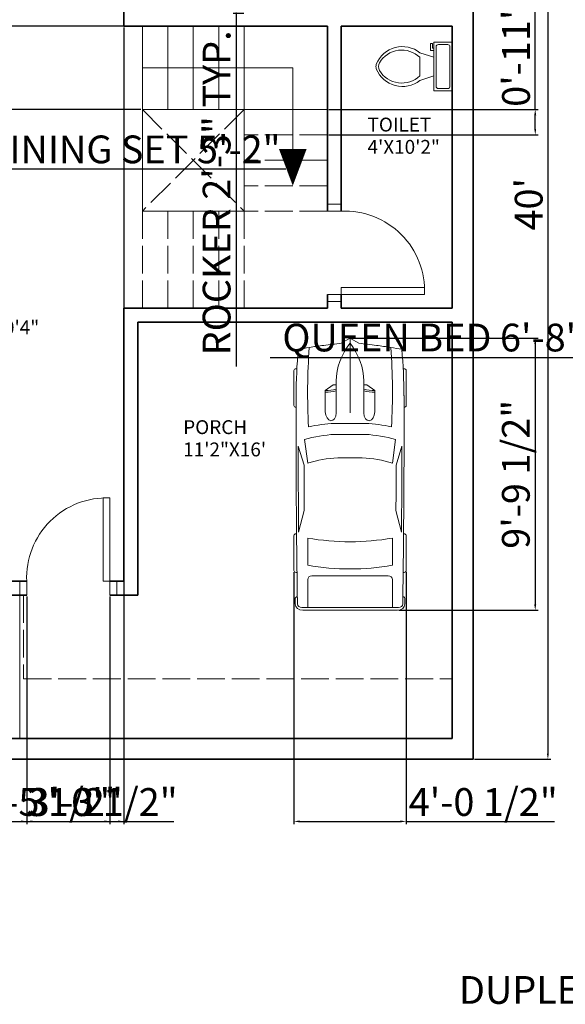
# Model space of a CAD drawing. Units: inches. Extents: x 2446 to 3341, y 462 to 1195.
# Tile 2 of 6: x 2649 to 2884, y 462 to 888. Entities that reach past the tile are written whole.
import ezdxf

# ---------------------------------------------------------------- set-up
doc = ezdxf.new("R2010")
doc.units = ezdxf.units.IN
doc.linetypes.add('ACAD_ISO02W100', pattern=[15, 12, -3])
for name, color, linetype, lineweight in [('A-ANNO-DIMS', 2, 'Continuous', 18), ('A-ANNO-TEXT', 7, 'Continuous', 25), ('A-AREA-IDEN', 7, 'Continuous', 18), ('A-DOOR', 4, 'Continuous', 18), ('A-FLOR-FIXT', 9, 'Continuous', 18), ('A-FLOR-HIDN', 8, 'ACAD_ISO02W100', 18), ('A-FLOR-STRS', 7, 'Continuous', 18), ('A-FLOR-STRS-HIDN', 8, 'ACAD_ISO02W100', 18), ('A-WALL', 7, 'Continuous', 35), ('C-PROP', 7, 'Continuous', 35), ('C-SITE-VEHC', 8, 'Continuous', 13), ('L-PLNT', 3, 'Continuous', 18)]:
    doc.layers.add(name, color=color, linetype=linetype, lineweight=lineweight)
doc.styles.get("Standard").update_dxf_attribs({"font": 'arial.ttf'})
doc.dimstyles.new('ISO-25', dxfattribs={"dimtxt": 12, "dimasz": 2.5, "dimexe": 1.25, "dimexo": 0.625, "dimtad": 1, "dimdec": 1, "dimlunit": 3, "dimtxsty": 'Standard', "dimcen": 2.5, "dimadec": 0, "dimazin": 0, "dimtfac": 1, "dimtdec": 1, "dimtmove": 0, "dimatfit": 3, "dimfxl": 1, "dimarcsym": 0})

# ---------------------------------------------------------------- blocks, each defined once
blk = doc.blocks.new('Toilet - top')
for p, q in [((9.5, -6), (9.5, -2)), ((-10, -8.5), (-8, -8.5)), ((-10, -9.5), (-10, -8.5)), ((-8, -8.5), (-8, -8)), ((-7, -8), (-7, -9.5)), ((-4, -8), (-6, -14)), ((4, -8), (6, -14)), ((-7, -9.5), (-10, -9.5)), ((4, -14), (-4, -14))]:
    blk.add_line(p, q)
blk.add_lwpolyline([(10.5, -8), (10.5, 0), (-10.5, 0), (-10.5, -8)], close=True)
for points in [[(-9.5, -2), (-9.5, -6)], [(8.5, -1), (-8.5, -1)], [(-8.5, -7), (8.5, -7)]]:
    blk.add_lwpolyline(points)
for centre, radius, start, end in [((-8.62, -1.88), 0.884, 81.8699, 188.1301), ((8.62, -1.88), 0.884, 351.8699, 98.1301), ((-8.62, -6.12), 0.884, 171.8699, 278.1301), ((8.62, -6.12), 0.884, 261.8699, 8.1301), ((3.52, -21.58), 12.17, 141.4691, 247.9714), ((4.2, -21.82), 11.33, 136.3677, 238.9468), ((-3.52, -21.58), 12.17, 292.0284, 38.5307), ((-4.2, -21.82), 11.33, 301.053, 43.6321), ((0, -27.88), 4, 245.7318, 294.2682), ((0, -29), 4, 254.8605, 285.1395)]:
    blk.add_arc(centre, radius, start, end)
blk = doc.blocks.new('*U14')
for p, q in [((21.1, 37.41), (21.1, 36.83)), ((46.55, 38.89), (22.35, 38.89)), ((47.8, 37.39), (47.8, 37.41)), ((87.99, 31.87), (74.76, 35.92)), ((134.31, 35.6), (119.29, 31.78)), ((135.45, 37.07), (135.45, 37.41)), ((136.7, 38.89), (160.9, 38.89)), ((162.15, 37.41), (162.15, 36.77)), ((70.03, 31.54), (86.41, 29.35)), ((138.42, 29.35), (157.25, 29.35)), ((186.47, 29.35), (167.01, 29.35)), ((186.47, -33.5), (186.47, 33.5)), ((188.4, -32.76), (188.4, 32.76)), ((164.52, 26.39), (164.52, -26.39)), ((32.27, 11.63), (36.13, 17.17)), ((36.13, 17.17), (50.94, 17.17)), ((29.77, 9.51), (51.68, 9.51)), ((32.12, 9.51), (32.12, 11.15)), ((58.92, -10.77), (58.92, 10.77)), ((66.55, -10.53), (66.55, 10.53)), ((82.74, 8.5), (82.74, -8.5)), ((186.47, -10.53), (186.47, 10.53)), ((3.27, 6.13), (0.1, 0.41)), ((0, 0), (51.68, 0)), ((0.1, -0.41), (3.27, -6.13)), ((29.77, -9.51), (51.68, -9.51)), ((32.12, -9.51), (32.12, -11.15)), ((32.27, -11.63), (36.13, -17.17)), ((36.13, -17.17), (50.94, -17.17)), ((86.41, -29.35), (70.03, -31.54)), ((87.99, -31.87), (74.76, -35.92)), ((134.31, -35.6), (119.29, -31.78)), ((157.25, -29.35), (138.42, -29.35)), ((167.01, -29.35), (186.47, -29.35)), ((21.1, -37.41), (21.1, -36.83)), ((46.55, -38.89), (22.35, -38.89)), ((47.8, -37.39), (47.8, -37.41)), ((135.45, -37.07), (135.45, -37.41)), ((136.7, -38.89), (160.9, -38.89)), ((162.15, -37.41), (162.15, -36.77))]:
    blk.add_line(p, q)
for centre, major_axis, ratio, start_param, end_param in [((266.03, -27.52), (0, 313.31), 0.842304, 1.367076, 1.39176), ((41.19, -490.86), (0, 528.23), 0.842304, 0.00281, 0.075598), ((22.35, 37.41), (0, -1.48), 0.842304, 3.141593, 4.712389), ((64.48, -10555.62), (0, 10593.03), 0.842304, -0.013397, 0.002797), ((46.55, 37.41), (0, 1.48), 0.842304, -1.570796, 0), ((64.48, -10555.62), (0, -10591.55), 0.842304, 3.133765, 3.140441), ((136.7, 37.41), (0, -1.48), 0.842304, 3.141593, 4.712389), ((160.9, 37.41), (0, 1.48), 0.842304, -1.570796, 0), ((180.63, 35.84), (0, 2.22), 0.842304, -0.013017, 1.249894), ((64.48, -10556.36), (0, 10595.31), 0.842304, -0.013397, -0.013017), ((183.98, 33.5), (0, -2.96), 0.842304, 1.570796, 3.128196), ((183.98, 32.76), (0, -5.25), 0.842304, 1.570796, 3.128196), ((259.18, -27.52), (0, -305.3), 0.842304, 4.528606, 4.561838), ((37.47, -593.96), (0, -623.33), 0.842304, 3.096046, 3.200911), ((134.4, 5.39), (0, -89.78), 0.842304, 4.449482, 4.652344), ((135.29, 5.39), (0, 81.77), 0.842304, 1.245306, 1.50788), ((149.6, 2.8), (0, -79.58), 0.842304, 4.372215, 4.640744), ((95.79, -3666.35), (0, -3698.24), 0.842304, 3.134049, 3.144098), ((17.08, 0), (0, 147.02), 0.842304, 4.511394, 4.913384), ((35.91, 0), (0, 147.02), 0.842304, 4.511394, 4.913384), ((167.01, 26.39), (0, 2.96), 0.842304, 0, 1.570796), ((-204.49, 52.4), (0, -250.96), 0.842304, 1.385369, 1.434372), ((13.04, 17.01), (0, 27.42), 0.842304, 4.435146, 4.718221), ((14.2, 17.01), (0, 27.42), 0.842304, 4.435146, 4.718221), ((50.79, 13.34), (6.34, -0.36), 0.603834, -1.395552, 1.581315), ((29.77, -46.66), (0, 56.17), 0.842304, 0, 0.590319), ((32.75, 11.15), (0, 0.74), 0.842304, 0.879714, 1.570796), ((0.62, 0), (0, -0.74), 0.842304, 4.131459, 5.293319), ((-204.49, -52.4), (0, 250.96), 0.842304, -1.434372, -1.385369), ((29.77, 46.66), (0, 56.17), 0.842304, 2.551274, 3.141593), ((32.75, -11.15), (0, -0.74), 0.842304, 4.712389, 5.403472), ((13.04, -17.01), (0, -27.42), 0.842304, 1.564964, 1.848039), ((14.2, -17.01), (0, -27.42), 0.842304, 1.564964, 1.848039), ((134.4, -5.39), (0, -89.78), 0.842304, -1.510751, -1.307889), ((135.29, -5.39), (0, -81.77), 0.842304, -1.50788, -1.245306), ((149.6, -2.8), (0, -79.58), 0.842304, -1.499151, -1.230623), ((259.18, 27.52), (0, 305.3), 0.842304, 1.721348, 1.754579), ((167.01, -26.39), (0, -2.96), 0.842304, 4.712389, 6.283185), ((266.03, 27.52), (0, 313.31), 0.842304, 1.749832, 1.774517), ((37.47, 593.96), (0, -623.33), 0.842304, -0.059319, 0.045547), ((95.79, 3666.35), (0, -3698.24), 0.842304, -0.002505, 0.007544), ((183.98, -33.5), (0, 2.96), 0.842304, 3.15499, 4.712389), ((183.98, -32.76), (0, -5.25), 0.842304, 0.013397, 1.570796), ((41.19, 490.86), (0, -528.23), 0.842304, -0.075598, -0.00281), ((22.35, -37.41), (0, 1.48), 0.842304, 1.570796, 3.141593), ((64.48, 10555.62), (0, 10593.03), 0.842304, 3.138796, 3.15499), ((46.55, -37.41), (0, -1.48), 0.842304, 0, 1.570796), ((64.48, 10555.62), (0, -10591.55), 0.842304, 0.001152, 0.007828), ((136.7, -37.41), (0, -1.48), 0.842304, -1.570796, 0), ((160.9, -37.41), (0, 1.48), 0.842304, 3.141593, 4.712389), ((180.63, -35.84), (0, -2.22), 0.842304, -1.249894, 0.013017), ((64.48, 10556.36), (0, 10595.31), 0.842304, 3.15461, 3.15499)]:
    blk.add_ellipse(centre, major_axis=major_axis, ratio=ratio, start_param=start_param, end_param=end_param)
at = {"extrusion": (0, 0, -1)}
blk.add_ellipse((50.79, -13.34), major_axis=(6.34, 0.36), ratio=0.603834, start_param=-1.395552, end_param=1.581315, dxfattribs=at)
blk = doc.blocks.new('*D18')
at = {"layer": 'A-ANNO-DIMS', "color": 0, "lineweight": -2, "transparency": 16777216}
for p, q in [((2845.24, 1047.97), (2878.2, 1047.97)), ((2876.95, 1045.47), (2876.95, 570.47)), ((2845.24, 567.97), (2878.2, 567.97))]:
    blk.add_line(p, q, dxfattribs=at)
at = {"layer": 'A-ANNO-DIMS', "color": 0, "transparency": 16777216}
for points in [[(2876.53, 1045.47), (2877.37, 1045.47), (2876.95, 1047.97)], [(2876.53, 570.47), (2877.37, 570.47), (2876.95, 567.97)]]:
    blk.add_solid(points, dxfattribs=at)
at = {"layer": 'Defpoints', "color": 0, "transparency": 16777216}
for p in [(2844.62, 1047.97), (2844.62, 567.97), (2876.95, 567.97)]:
    blk.add_point(p, dxfattribs=at)
at = {"layer": 'A-ANNO-DIMS', "color": 0, "transparency": 16777216, "insert": (2870.2, 807.97), "char_height": 12, "attachment_point": 5, "rotation": 90}
blk.add_mtext("40'", dxfattribs=at)
blk = doc.blocks.new('DOOR-SWING-36IN')
for p, q in [((6, 42), (0, 42)), ((6, 39), (0, 39)), ((6, 3), (0, 3)), ((6, 0), (0, 0))]:
    blk.add_line(p, q)
blk.add_lwpolyline([(6, 3), (42, 3), (42, 6), (6, 6)], close=True)
blk.add_arc((7.5, 4.5), 34.53, 357.5104, 92.4896)
blk = doc.blocks.new('*D29')
at = {"layer": 'A-ANNO-DIMS', "color": 0, "lineweight": -2, "transparency": 16777216}
for p, q in [((2937.19, 741.58), (2756.92, 741.58)), ((2937.19, 730.2), (2937.19, 742.83)), ((3014.69, 741.58), (2939.69, 741.58)), ((3017.19, 730.2), (3017.19, 742.83))]:
    blk.add_line(p, q, dxfattribs=at)
at = {"layer": 'A-ANNO-DIMS', "color": 0, "transparency": 16777216}
for points in [[(2939.69, 742), (2939.69, 741.16), (2937.19, 741.58)], [(3014.69, 742), (3014.69, 741.16), (3017.19, 741.58)]]:
    blk.add_solid(points, dxfattribs=at)
at = {"layer": 'Defpoints', "color": 0, "transparency": 16777216}
for p in [(2937.19, 741.58), (2937.19, 729.58), (3017.19, 729.58)]:
    blk.add_point(p, dxfattribs=at)
at = {"layer": 'A-ANNO-DIMS', "color": 0, "transparency": 16777216, "insert": (2845.81, 748.78), "char_height": 12, "attachment_point": 5}
blk.add_mtext('QUEEN BED 6\'-8" TYP.', dxfattribs=at)
blk = doc.blocks.new('*D33')
at = {"layer": 'A-ANNO-DIMS', "color": 0, "lineweight": -2, "transparency": 16777216}
for p, q in [((2745.53, 917.47), (2740.86, 917.47)), ((2742.11, 914.97), (2742.11, 892.97)), ((2745.53, 890.47), (2740.86, 890.47)), ((2742.11, 890.47), (2742.11, 737.82))]:
    blk.add_line(p, q, dxfattribs=at)
at = {"layer": 'A-ANNO-DIMS', "color": 0, "transparency": 16777216}
for points in [[(2741.69, 914.97), (2742.53, 914.97), (2742.11, 917.47)], [(2741.69, 892.97), (2742.53, 892.97), (2742.11, 890.47)]]:
    blk.add_solid(points, dxfattribs=at)
at = {"layer": 'Defpoints', "color": 0, "transparency": 16777216}
for p in [(2746.16, 917.47), (2742.11, 890.47), (2746.16, 890.47)]:
    blk.add_point(p, dxfattribs=at)
at = {"layer": 'A-ANNO-DIMS', "color": 0, "transparency": 16777216, "insert": (2735.27, 812.89), "char_height": 12, "attachment_point": 5, "rotation": 90}
blk.add_mtext('ROCKER 2\'-3" TYP.', dxfattribs=at)
blk = doc.blocks.new('*D53')
at = {"layer": 'A-ANNO-DIMS', "color": 0, "lineweight": -2, "transparency": 16777216}
for p, q in [((2566.04, 831.98), (2566.04, 822.05)), ((2628.06, 831.98), (2628.06, 822.05)), ((2568.54, 823.3), (2625.56, 823.3)), ((2628.06, 823.3), (2763.7, 823.3))]:
    blk.add_line(p, q, dxfattribs=at)
at = {"layer": 'A-ANNO-DIMS', "color": 0, "transparency": 16777216}
for points in [[(2568.54, 823.72), (2568.54, 822.89), (2566.04, 823.3)], [(2625.56, 823.72), (2625.56, 822.89), (2628.06, 823.3)]]:
    blk.add_solid(points, dxfattribs=at)
at = {"layer": 'Defpoints', "color": 0, "transparency": 16777216}
for p in [(2566.04, 832.6), (2628.06, 832.6), (2628.06, 823.3)]:
    blk.add_point(p, dxfattribs=at)
at = {"layer": 'A-ANNO-DIMS', "color": 0, "transparency": 16777216, "insert": (2697.13, 830.13), "char_height": 12, "attachment_point": 5}
blk.add_mtext('DINING SET 5\'-2"', dxfattribs=at)
blk = doc.blocks.new('*D62')
at = {"layer": 'A-ANNO-DIMS', "color": 0, "lineweight": -2, "transparency": 16777216}
for p, q in [((2871.47, 848.97), (2871.47, 893.94)), ((2782.24, 848.97), (2872.72, 848.97)), ((2871.47, 840.47), (2871.47, 846.47)), ((2782.24, 837.97), (2872.72, 837.97))]:
    blk.add_line(p, q, dxfattribs=at)
at = {"layer": 'A-ANNO-DIMS', "color": 0, "transparency": 16777216}
for points in [[(2871.05, 846.47), (2871.88, 846.47), (2871.47, 848.97)], [(2871.05, 840.47), (2871.88, 840.47), (2871.47, 837.97)]]:
    blk.add_solid(points, dxfattribs=at)
at = {"layer": 'Defpoints', "color": 0, "transparency": 16777216}
for p in [(2781.62, 848.97), (2871.47, 848.97), (2781.62, 837.97)]:
    blk.add_point(p, dxfattribs=at)
at = {"layer": 'A-ANNO-DIMS', "color": 0, "transparency": 16777216, "insert": (2864.71, 872.71), "char_height": 12, "attachment_point": 5, "rotation": 90}
blk.add_mtext('0\'-11"', dxfattribs=at)
blk = doc.blocks.new('*D63')
at = {"layer": 'A-ANNO-DIMS', "color": 0, "lineweight": -2, "transparency": 16777216}
for p, q in [((2700.99, 884.97), (2516.52, 884.97)), ((2517.77, 882.47), (2517.77, 851.47)), ((2700.99, 848.97), (2516.52, 848.97))]:
    blk.add_line(p, q, dxfattribs=at)
at = {"layer": 'A-ANNO-DIMS', "color": 0, "transparency": 16777216}
for points in [[(2517.35, 882.47), (2518.18, 882.47), (2517.77, 884.97)], [(2517.35, 851.47), (2518.18, 851.47), (2517.77, 848.97)]]:
    blk.add_solid(points, dxfattribs=at)
at = {"layer": 'Defpoints', "color": 0, "transparency": 16777216}
for p in [(2701.62, 884.97), (2517.77, 848.97), (2701.62, 848.97)]:
    blk.add_point(p, dxfattribs=at)
at = {"layer": 'A-ANNO-DIMS', "color": 0, "transparency": 16777216, "insert": (2511.01, 866.97), "char_height": 12, "attachment_point": 5, "rotation": 90}
blk.add_mtext('3\'-0"', dxfattribs=at)
blk = doc.blocks.new('*D72')
at = {"layer": 'A-ANNO-DIMS', "color": 0, "lineweight": -2, "transparency": 16777216}
for p, q in [((2612.15, 638.34), (2612.15, 539.87)), ((2651.62, 638.34), (2651.62, 539.87)), ((2614.65, 541.12), (2649.12, 541.12)), ((2651.62, 541.12), (2715.22, 541.12))]:
    blk.add_line(p, q, dxfattribs=at)
at = {"layer": 'A-ANNO-DIMS', "color": 0, "transparency": 16777216}
for points in [[(2614.65, 541.54), (2614.65, 540.7), (2612.15, 541.12)], [(2649.12, 541.54), (2649.12, 540.7), (2651.62, 541.12)]]:
    blk.add_solid(points, dxfattribs=at)
at = {"layer": 'Defpoints', "color": 0, "transparency": 16777216}
for p in [(2612.15, 638.97), (2651.62, 638.97), (2651.62, 541.12)]:
    blk.add_point(p, dxfattribs=at)
at = {"layer": 'A-ANNO-DIMS', "color": 0, "transparency": 16777216, "insert": (2684.67, 547.95), "char_height": 12, "attachment_point": 5}
blk.add_mtext('3\'-3 1/2"', dxfattribs=at)
blk = doc.blocks.new('*D73')
at = {"layer": 'A-ANNO-DIMS', "color": 0, "lineweight": -2, "transparency": 16777216}
for p, q in [((2651.62, 638.34), (2651.62, 539.87)), ((2687.62, 638.34), (2687.62, 539.87)), ((2654.12, 541.12), (2685.12, 541.12))]:
    blk.add_line(p, q, dxfattribs=at)
at = {"layer": 'A-ANNO-DIMS', "color": 0, "transparency": 16777216}
for points in [[(2654.12, 541.54), (2654.12, 540.7), (2651.62, 541.12)], [(2685.12, 541.54), (2685.12, 540.7), (2687.62, 541.12)]]:
    blk.add_solid(points, dxfattribs=at)
at = {"layer": 'Defpoints', "color": 0, "transparency": 16777216}
for p in [(2651.62, 638.97), (2687.62, 638.97), (2687.62, 541.12)]:
    blk.add_point(p, dxfattribs=at)
at = {"layer": 'A-ANNO-DIMS', "color": 0, "transparency": 16777216, "insert": (2669.62, 547.88), "char_height": 12, "attachment_point": 5}
blk.add_mtext('3\'-0"', dxfattribs=at)
blk = doc.blocks.new('*D74')
at = {"layer": 'A-ANNO-DIMS', "color": 0, "lineweight": -2, "transparency": 16777216}
for p, q in [((2628.27, 884.34), (2628.27, 539.87)), ((2693.62, 884.34), (2693.62, 539.87)), ((2630.77, 541.12), (2691.12, 541.12))]:
    blk.add_line(p, q, dxfattribs=at)
at = {"layer": 'A-ANNO-DIMS', "color": 0, "transparency": 16777216}
for points in [[(2630.77, 541.54), (2630.77, 540.7), (2628.27, 541.12)], [(2691.12, 541.54), (2691.12, 540.7), (2693.62, 541.12)]]:
    blk.add_solid(points, dxfattribs=at)
at = {"layer": 'Defpoints', "color": 0, "transparency": 16777216}
for p in [(2628.27, 884.97), (2693.62, 884.97), (2693.62, 541.12)]:
    blk.add_point(p, dxfattribs=at)
at = {"layer": 'A-ANNO-DIMS', "color": 0, "transparency": 16777216, "insert": (2660.94, 547.95), "char_height": 12, "attachment_point": 5}
blk.add_mtext('5\'-5 1/2"', dxfattribs=at)
blk = doc.blocks.new('*D84')
at = {"layer": 'A-ANNO-DIMS', "color": 0, "lineweight": -2, "transparency": 16777216}
for p, q in [((2767.14, 648.95), (2767.14, 539.87)), ((2815.68, 648.95), (2815.68, 539.87)), ((2769.64, 541.12), (2813.18, 541.12)), ((2815.68, 541.12), (2879.78, 541.12))]:
    blk.add_line(p, q, dxfattribs=at)
at = {"layer": 'A-ANNO-DIMS', "color": 0, "transparency": 16777216}
for points in [[(2769.64, 541.54), (2769.64, 540.7), (2767.14, 541.12)], [(2813.18, 541.54), (2813.18, 540.7), (2815.68, 541.12)]]:
    blk.add_solid(points, dxfattribs=at)
at = {"layer": 'Defpoints', "color": 0, "transparency": 16777216}
for p in [(2767.14, 649.57), (2815.68, 649.57), (2815.68, 541.12)]:
    blk.add_point(p, dxfattribs=at)
at = {"layer": 'A-ANNO-DIMS', "color": 0, "transparency": 16777216, "insert": (2848.98, 547.95), "char_height": 12, "attachment_point": 5}
blk.add_mtext('4\'-0 1/2"', dxfattribs=at)
blk = doc.blocks.new('*D85')
at = {"layer": 'A-ANNO-DIMS', "color": 0, "lineweight": -2, "transparency": 16777216}
for p, q in [((2792.03, 750), (2872.72, 750)), ((2871.47, 747.5), (2871.47, 634.91)), ((2812.48, 632.41), (2872.72, 632.41))]:
    blk.add_line(p, q, dxfattribs=at)
at = {"layer": 'A-ANNO-DIMS', "color": 0, "transparency": 16777216}
for points in [[(2871.05, 747.5), (2871.88, 747.5), (2871.47, 750)], [(2871.05, 634.91), (2871.88, 634.91), (2871.47, 632.41)]]:
    blk.add_solid(points, dxfattribs=at)
at = {"layer": 'Defpoints', "color": 0, "transparency": 16777216}
for p in [(2791.41, 750), (2811.86, 632.41), (2871.47, 632.41)]:
    blk.add_point(p, dxfattribs=at)
at = {"layer": 'A-ANNO-DIMS', "color": 0, "transparency": 16777216, "insert": (2864.64, 691.2), "char_height": 12, "attachment_point": 5, "rotation": 90}
blk.add_mtext('9\'-9 1/2"', dxfattribs=at)

msp = doc.modelspace()

# ---------------------------------------------------------------- linework, layer by layer
at = {"layer": 'A-FLOR-HIDN'}
for p, q in [((2650.28, 638.97), (2650.28, 602.7)), ((2650.28, 602.7), (2835.62, 602.7))]:
    msp.add_line(p, q, dxfattribs=at)
at = {"layer": 'A-FLOR-STRS'}
for p, q in [((2701.62, 848.97), (2701.62, 884.97)), ((2712.62, 848.97), (2712.62, 884.97)), ((2723.62, 848.97), (2723.62, 884.97)), ((2734.62, 848.97), (2734.62, 884.97)), ((2745.62, 804.97), (2745.62, 884.97)), ((2781.62, 848.97), (2701.62, 848.97)), ((2701.62, 804.97), (2701.62, 848.97)), ((2745.62, 804.97), (2701.62, 804.97))]:
    msp.add_line(p, q, dxfattribs=at)
msp.add_lwpolyline([(2701.62, 866.97), (2766.66, 866.97), (2766.66, 831.9)], dxfattribs=at)
msp.add_lwpolyline([(2766.66, 831.9, 12, 0, 0), (2766.66, 815.97, 0, 0, 0)], format="xyseb", dxfattribs=at)
at = {"layer": 'A-FLOR-STRS-HIDN'}
for p, q in [((2701.62, 848.97), (2745.62, 804.97)), ((2745.62, 848.97), (2701.62, 804.97)), ((2781.62, 837.97), (2745.62, 837.97)), ((2781.62, 826.97), (2745.62, 826.97)), ((2781.62, 815.97), (2745.62, 815.97)), ((2701.62, 762.97), (2701.62, 804.97)), ((2712.62, 762.97), (2712.62, 804.97)), ((2723.62, 762.97), (2723.62, 804.97)), ((2734.62, 762.97), (2734.62, 804.97)), ((2781.62, 804.97), (2745.62, 804.97)), ((2745.62, 804.97), (2745.62, 762.97))]:
    msp.add_line(p, q, dxfattribs=at)
at = {"layer": 'A-WALL'}
for p, q in [((2693.62, 890.97), (2693.62, 884.97)), ((2699.62, 884.97), (2693.62, 884.97)), ((2781.62, 884.97), (2699.62, 884.97)), ((2781.62, 804.97), (2781.62, 884.97)), ((2835.62, 884.97), (2787.62, 884.97)), ((2787.62, 804.97), (2787.62, 884.97)), ((2835.62, 762.97), (2835.62, 884.97)), ((2781.62, 762.97), (2781.62, 768.97)), ((2787.62, 762.97), (2787.62, 768.97)), ((2693.62, 762.97), (2693.62, 644.97)), ((2699.62, 762.97), (2693.62, 762.97)), ((2781.62, 762.97), (2699.62, 762.97)), ((2835.62, 762.97), (2787.62, 762.97)), ((2835.62, 756.97), (2699.62, 756.97)), ((2699.62, 756.97), (2699.62, 638.97)), ((2835.62, 576.97), (2835.62, 756.97)), ((2651.62, 644.97), (2553.62, 644.97)), ((2693.62, 644.97), (2687.62, 644.97)), ((2651.62, 638.97), (2553.62, 638.97)), ((2693.62, 638.97), (2687.62, 638.97)), ((2693.62, 638.97), (2699.62, 638.97)), ((2553.62, 576.97), (2693.62, 576.97)), ((2648.62, 576.97), (2835.62, 576.97))]:
    msp.add_line(p, q, dxfattribs=at)
at = {"layer": 'C-PROP'}
msp.add_lwpolyline([(2544.62, 567.97), (2844.62, 567.97), (2844.62, 1047.97), (2544.62, 1047.97)], close=True, dxfattribs=at)
at = {"layer": 'L-PLNT'}
msp.add_line((2648.62, 638.97), (2648.62, 576.97), dxfattribs=at)

# ---------------------------------------------------------------- block references
at = {"layer": 'A-DOOR'}
msp.add_blockref('DOOR-SWING-36IN', (2781.62, 765.97), dxfattribs=at)
at = {"layer": 'A-DOOR', "rotation": 89.99999999999883}
msp.add_blockref('DOOR-SWING-36IN', (2690.62, 638.97), dxfattribs=at)
at = {"layer": 'A-FLOR-FIXT', "rotation": 270}
msp.add_blockref('Toilet - top', (2835.62, 867.49), dxfattribs=at)
at = {"layer": 'C-SITE-VEHC', "xscale": 0.6241911502922983, "yscale": 0.6241911502922983, "zscale": 0.6241911502922983, "rotation": 270.0000000000023}
msp.add_blockref('*U14', (2791.41, 750), dxfattribs=at)

# ---------------------------------------------------------------- texts
at = {"layer": 'A-ANNO-TEXT'}
msp.add_text('DUPLEX HOUSE', height=12, dxfattribs=at).set_placement((2838.48, 462.25))
at = {"layer": 'A-AREA-IDEN'}
for s, p in [('TOILET', (2798.97, 839.41)), ('4\'X10\'2"', (2798.97, 829.77)), ('11\'8"X20\'4"', (2612.78, 751.71)), ('PORCH', (2719.28, 708.59)), ('11\'2"X16\'', (2719.28, 698.95))]:
    msp.add_text(s, height=6, dxfattribs=at).set_placement(p)

# ---------------------------------------------------------------- dimensions: what is measured, and where the dimension line sits
at = {"layer": 'A-ANNO-DIMS'}
for base, p1, p2, override, picture, middle in [((2876.95, 567.97), (2844.62, 1047.97), (2844.62, 567.97), {"dimclrd": 0, "dimclre": 0, "dimclrt": 0}, '*D18', (2870.2, 807.97)), ((2871.47, 848.97), (2781.62, 837.97), (2781.62, 848.97), {"dimdec": 1, "dimlfac": 1, "dimrnd": 0, "dimzin": 1, "dimdsep": 46, "dimlunit": 4, "dimfrac": 2}, '*D62', (2864.71, 872.71)), ((2517.77, 848.97), (2701.62, 884.97), (2701.62, 848.97), {"dimdec": 1, "dimlfac": 1, "dimrnd": 0, "dimzin": 1, "dimdsep": 46, "dimlunit": 4, "dimfrac": 2}, '*D63', (2511.01, 866.97)), ((2871.47, 632.41), (2791.41, 750), (2811.86, 632.41), {"dimdec": 1, "dimlfac": 1, "dimrnd": 0, "dimzin": 1, "dimdsep": 46, "dimlunit": 4, "dimfrac": 2}, '*D85', (2864.64, 691.2))]:
    dim = msp.add_linear_dim(base=base, p1=p1, p2=p2, angle=90, dimstyle='ISO-25', override=override, dxfattribs=at)
    dim.commit()
    dim.dimension.update_dxf_attribs({"geometry": picture, "text_midpoint": middle})
for base, p1, p2, angle, text, picture, middle in [((2742.11, 890.47), (2746.16, 917.47), (2746.16, 890.47), 270, 'ROCKER <> TYP.', '*D33', (2735.27, 812.89)), ((2937.19, 741.58), (3017.19, 729.58), (2937.19, 729.58), 180, 'QUEEN BED <> TYP.', '*D29', (2845.81, 748.78))]:
    dim = msp.add_linear_dim(base=base, p1=p1, p2=p2, angle=angle, text=text, dimstyle='ISO-25', override={"dimdec": 1, "dimlfac": 1, "dimrnd": 0, "dimzin": 1, "dimdsep": 46, "dimlunit": 4, "dimfrac": 2}, dxfattribs=at)
    dim.commit()
    dim.dimension.update_dxf_attribs({"geometry": picture, "text_midpoint": middle})
for base, p1, p2, picture, middle in [((2693.6165, 541.1195), (2628.2718, 884.9695), (2693.6165, 884.9695), '*D74', (2660.9442, 547.9492)), ((2815.68, 541.12), (2767.14, 649.57), (2815.68, 649.57), '*D84', (2848.98, 547.95)), ((2651.62, 541.12), (2612.15, 638.97), (2651.62, 638.97), '*D72', (2684.67, 547.95)), ((2687.62, 541.12), (2651.62, 638.97), (2687.62, 638.97), '*D73', (2669.62, 547.88))]:
    dim = msp.add_linear_dim(base=base, p1=p1, p2=p2, dimstyle='ISO-25', override={"dimdec": 1, "dimlfac": 1, "dimrnd": 0, "dimzin": 1, "dimdsep": 46, "dimlunit": 4, "dimfrac": 2}, dxfattribs=at)
    dim.commit()
    dim.dimension.update_dxf_attribs({"geometry": picture, "text_midpoint": middle})
dim = msp.add_linear_dim(base=(2628.06, 823.3), p1=(2566.04, 832.6), p2=(2628.06, 832.6), text='DINING SET <>', dimstyle='ISO-25', override={"dimdec": 1, "dimlfac": 1, "dimrnd": 0, "dimzin": 1, "dimdsep": 46, "dimlunit": 4, "dimfrac": 2}, dxfattribs=at)
dim.commit()
dim.dimension.update_dxf_attribs({"geometry": '*D53', "text_midpoint": (2697.13, 830.13)})

doc.saveas('drawing.dxf')
